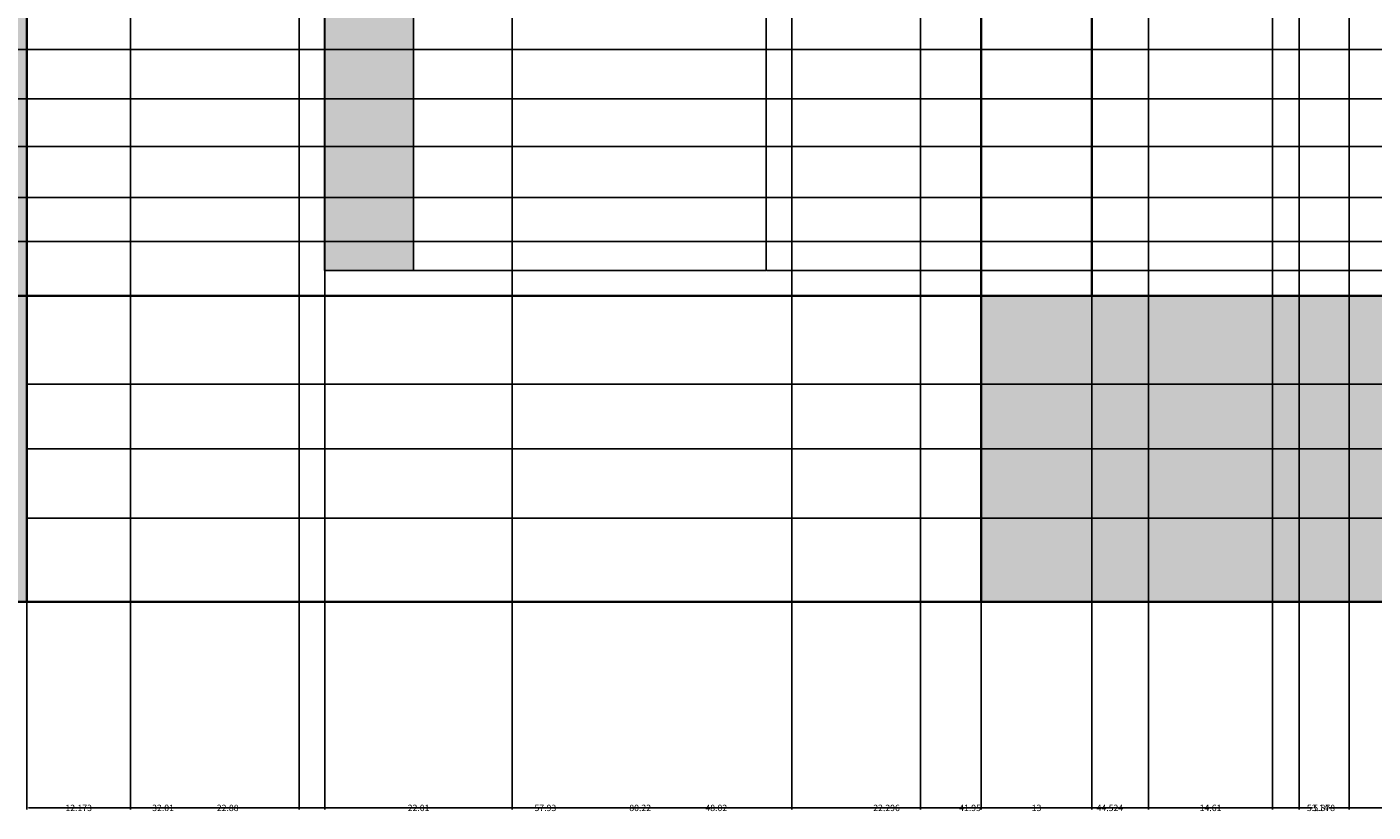
# Model space of a CAD drawing. Units: inches. Extents: x 62 to 566, y 66 to 528.
# Tile 11 of 20: x 284 to 443, y 66 to 158. Entities that reach past the tile are written whole.
import ezdxf

# ---------------------------------------------------------------- set-up
doc = ezdxf.new("R2010")
doc.units = ezdxf.units.IN
doc.header["$MEASUREMENT"] = 0
for name, color, linetype, lineweight in [('A-ANNO-DIMS', 2, 'Continuous', 18), ('A-DOOR', 4, 'Continuous', 25), ('A-ELEV', 7, 'Continuous', 35), ('A-FLOR-STRS', 2, 'Continuous', 25), ('A-WALL-PATT', 8, 'Continuous', 13)]:
    doc.layers.add(name, color=color, linetype=linetype, lineweight=lineweight)
doc.styles.get("Standard").update_dxf_attribs({"font": 'arial.ttf'})
doc.dimstyles.get("Standard").update_dxf_attribs({"dimtxt": 0.75, "dimasz": 0.18, "dimexe": 0.18, "dimexo": 0.0625, "dimgap": 0.09, "dimtad": 0, "dimtih": 1, "dimtoh": 1, "dimdec": 4, "dimzin": 0, "dimdsep": 46, "dimlunit": 4, "dimtxsty": 'Standard', "dimcen": 0.09, "dimadec": 0, "dimazin": 0, "dimtfac": 1, "dimtdec": 4, "dimtofl": 0, "dimtmove": 0, "dimatfit": 3, "dimfxl": 1, "dimtolj": 1, "dimtzin": 0, "dimarcsym": 0})

# ---------------------------------------------------------------- blocks, each defined once
blk = doc.blocks.new('*D9')
at = {"layer": 'A-ANNO-DIMS', "color": 0, "lineweight": -2, "transparency": 16777216}
for p, q in [((284.2, 271.35), (284.2, 65.94)), ((316.21, 126.31), (316.21, 65.94)), ((284.38, 66.12), (298.92, 66.12)), ((316.03, 66.12), (301.49, 66.12))]:
    blk.add_line(p, q, dxfattribs=at)
at = {"layer": 'A-ANNO-DIMS', "color": 0, "transparency": 16777216}
for points in [[(284.38, 66.15), (284.38, 66.09), (284.2, 66.12)], [(316.03, 66.15), (316.03, 66.09), (316.21, 66.12)]]:
    blk.add_solid(points, dxfattribs=at)
at = {"layer": 'Defpoints', "color": 0, "transparency": 16777216}
for p in [(284.2, 271.41), (316.21, 126.37), (316.21, 66.12)]:
    blk.add_point(p, dxfattribs=at)
at = {"layer": 'A-ANNO-DIMS', "color": 0, "transparency": 16777216, "insert": (300.21, 66.12), "char_height": 0.75, "attachment_point": 5}
blk.add_mtext('\\A1;32.01', dxfattribs=at)
blk = doc.blocks.new('*D10')
at = {"layer": 'A-ANNO-DIMS', "color": 0, "lineweight": -2, "transparency": 16777216}
for p, q in [((396.43, 271.35), (396.43, 65.94)), ((316.21, 126.31), (316.21, 65.94)), ((316.39, 66.12), (354.97, 66.12)), ((396.25, 66.12), (357.67, 66.12))]:
    blk.add_line(p, q, dxfattribs=at)
at = {"layer": 'A-ANNO-DIMS', "color": 0, "transparency": 16777216}
for points in [[(316.39, 66.15), (316.39, 66.09), (316.21, 66.12)], [(396.25, 66.15), (396.25, 66.09), (396.43, 66.12)]]:
    blk.add_solid(points, dxfattribs=at)
at = {"layer": 'Defpoints', "color": 0, "transparency": 16777216}
for p in [(396.43, 271.41), (316.21, 126.37), (396.43, 66.12)]:
    blk.add_point(p, dxfattribs=at)
at = {"layer": 'A-ANNO-DIMS', "color": 0, "transparency": 16777216, "insert": (356.32, 66.12), "char_height": 0.75, "attachment_point": 5}
blk.add_mtext('\\A1;80.22', dxfattribs=at)
blk = doc.blocks.new('*D11')
at = {"layer": 'A-ANNO-DIMS', "color": 0, "lineweight": -2, "transparency": 16777216}
for p, q in [((396.43, 271.35), (396.43, 65.94)), ((409.43, 126.31), (409.43, 65.94)), ((396.61, 66.12), (402.34, 66.12)), ((409.25, 66.12), (403.52, 66.12))]:
    blk.add_line(p, q, dxfattribs=at)
at = {"layer": 'A-ANNO-DIMS', "color": 0, "transparency": 16777216}
for points in [[(396.61, 66.15), (396.61, 66.09), (396.43, 66.12)], [(409.25, 66.15), (409.25, 66.09), (409.43, 66.12)]]:
    blk.add_solid(points, dxfattribs=at)
at = {"layer": 'Defpoints', "color": 0, "transparency": 16777216}
for p in [(396.43, 271.41), (409.43, 126.37), (409.43, 66.12)]:
    blk.add_point(p, dxfattribs=at)
at = {"layer": 'A-ANNO-DIMS', "color": 0, "transparency": 16777216, "insert": (402.93, 66.12), "char_height": 0.75, "attachment_point": 5}
blk.add_mtext('\\A1;13', dxfattribs=at)
blk = doc.blocks.new('*D12')
at = {"layer": 'A-ANNO-DIMS', "color": 0, "lineweight": -2, "transparency": 16777216}
for p, q in [((409.43, 126.31), (409.43, 65.94)), ((462.58, 126.31), (462.58, 65.94)), ((409.61, 66.12), (434.65, 66.12)), ((462.4, 66.12), (437.36, 66.12))]:
    blk.add_line(p, q, dxfattribs=at)
at = {"layer": 'A-ANNO-DIMS', "color": 0, "transparency": 16777216}
for points in [[(409.61, 66.15), (409.61, 66.09), (409.43, 66.12)], [(462.4, 66.15), (462.4, 66.09), (462.58, 66.12)]]:
    blk.add_solid(points, dxfattribs=at)
at = {"layer": 'Defpoints', "color": 0, "transparency": 16777216}
for p in [(409.43, 126.37), (462.58, 126.37), (462.58, 66.12)]:
    blk.add_point(p, dxfattribs=at)
at = {"layer": 'A-ANNO-DIMS', "color": 0, "transparency": 16777216, "insert": (436, 66.12), "char_height": 0.75, "attachment_point": 5}
blk.add_mtext('\\A1;53.14', dxfattribs=at)
blk = doc.blocks.new('*D40')
at = {"layer": 'A-ANNO-DIMS', "color": 0, "lineweight": -2, "transparency": 16777216}
for p, q in [((284.2, 445.04), (284.2, 65.94)), ((316.21, 417.64), (316.21, 65.94)), ((284.38, 66.12), (298.92, 66.12)), ((316.03, 66.12), (301.49, 66.12))]:
    blk.add_line(p, q, dxfattribs=at)
at = {"layer": 'A-ANNO-DIMS', "color": 0, "transparency": 16777216}
for points in [[(284.38, 66.15), (284.38, 66.09), (284.2, 66.12)], [(316.03, 66.15), (316.03, 66.09), (316.21, 66.12)]]:
    blk.add_solid(points, dxfattribs=at)
at = {"layer": 'Defpoints', "color": 0, "transparency": 16777216}
for p in [(284.2, 445.11), (316.21, 417.71), (316.21, 66.12)]:
    blk.add_point(p, dxfattribs=at)
at = {"layer": 'A-ANNO-DIMS', "color": 0, "transparency": 16777216, "insert": (300.21, 66.12), "char_height": 0.75, "attachment_point": 5}
blk.add_mtext('\\A1;32.01', dxfattribs=at)
blk = doc.blocks.new('*D41')
at = {"layer": 'A-ANNO-DIMS', "color": 0, "lineweight": -2, "transparency": 16777216}
for p, q in [((316.21, 417.64), (316.21, 65.94)), ((374.14, 417.64), (374.14, 65.94)), ((316.39, 66.12), (343.82, 66.12)), ((373.96, 66.12), (346.53, 66.12))]:
    blk.add_line(p, q, dxfattribs=at)
at = {"layer": 'A-ANNO-DIMS', "color": 0, "transparency": 16777216}
for points in [[(316.39, 66.15), (316.39, 66.09), (316.21, 66.12)], [(373.96, 66.15), (373.96, 66.09), (374.14, 66.12)]]:
    blk.add_solid(points, dxfattribs=at)
at = {"layer": 'Defpoints', "color": 0, "transparency": 16777216}
for p in [(316.21, 417.71), (374.14, 417.71), (374.14, 66.12)]:
    blk.add_point(p, dxfattribs=at)
at = {"layer": 'A-ANNO-DIMS', "color": 0, "transparency": 16777216, "insert": (345.17, 66.12), "char_height": 0.75, "attachment_point": 5}
blk.add_mtext('\\A1;57.93', dxfattribs=at)
blk = doc.blocks.new('*D42')
at = {"layer": 'A-ANNO-DIMS', "color": 0, "lineweight": -2, "transparency": 16777216}
for p, q in [((416.08, 445.04), (416.08, 65.94)), ((374.14, 417.64), (374.14, 65.94)), ((374.32, 66.12), (393.74, 66.12)), ((415.9, 66.12), (396.48, 66.12))]:
    blk.add_line(p, q, dxfattribs=at)
at = {"layer": 'A-ANNO-DIMS', "color": 0, "transparency": 16777216}
for points in [[(374.32, 66.15), (374.32, 66.09), (374.14, 66.12)], [(415.9, 66.15), (415.9, 66.09), (416.08, 66.12)]]:
    blk.add_solid(points, dxfattribs=at)
at = {"layer": 'Defpoints', "color": 0, "transparency": 16777216}
for p in [(416.08, 445.11), (374.14, 417.71), (416.08, 66.12)]:
    blk.add_point(p, dxfattribs=at)
at = {"layer": 'A-ANNO-DIMS', "color": 0, "transparency": 16777216, "insert": (395.11, 66.12), "char_height": 0.75, "attachment_point": 5}
blk.add_mtext('\\A1;41.95', dxfattribs=at)
blk = doc.blocks.new('*D43')
at = {"layer": 'A-ANNO-DIMS', "color": 0, "lineweight": -2, "transparency": 16777216}
for p, q in [((416.08, 445.04), (416.08, 65.94)), ((430.69, 445.04), (430.69, 65.94)), ((416.26, 66.12), (422.14, 66.12)), ((430.51, 66.12), (424.64, 66.12))]:
    blk.add_line(p, q, dxfattribs=at)
at = {"layer": 'A-ANNO-DIMS', "color": 0, "transparency": 16777216}
for points in [[(416.26, 66.15), (416.26, 66.09), (416.08, 66.12)], [(430.51, 66.15), (430.51, 66.09), (430.69, 66.12)]]:
    blk.add_solid(points, dxfattribs=at)
at = {"layer": 'Defpoints', "color": 0, "transparency": 16777216}
for p in [(416.08, 445.11), (430.69, 445.11), (430.69, 66.12)]:
    blk.add_point(p, dxfattribs=at)
at = {"layer": 'A-ANNO-DIMS', "color": 0, "transparency": 16777216, "insert": (423.39, 66.12), "char_height": 0.75, "attachment_point": 5}
blk.add_mtext('\\A1;14.61', dxfattribs=at)
blk = doc.blocks.new('*D57')
at = {"layer": 'A-ANNO-DIMS', "color": 0, "lineweight": -2, "transparency": 16777216}
for p, q in [((316.21, 126.31), (316.21, 65.94)), ((284.2, 90.31), (284.2, 65.94)), ((284.38, 66.12), (298.92, 66.12)), ((316.03, 66.12), (301.49, 66.12))]:
    blk.add_line(p, q, dxfattribs=at)
at = {"layer": 'A-ANNO-DIMS', "color": 0, "transparency": 16777216}
for points in [[(284.38, 66.15), (284.38, 66.09), (284.2, 66.12)], [(316.03, 66.15), (316.03, 66.09), (316.21, 66.12)]]:
    blk.add_solid(points, dxfattribs=at)
at = {"layer": 'Defpoints', "color": 0, "transparency": 16777216}
for p in [(316.21, 126.37), (284.2, 90.37), (316.21, 66.12)]:
    blk.add_point(p, dxfattribs=at)
at = {"layer": 'A-ANNO-DIMS', "color": 0, "transparency": 16777216, "insert": (300.21, 66.12), "char_height": 0.75, "attachment_point": 5}
blk.add_mtext('\\A1;32.01', dxfattribs=at)
blk = doc.blocks.new('*D58')
at = {"layer": 'A-ANNO-DIMS', "color": 0, "lineweight": -2, "transparency": 16777216}
for p, q in [((316.21, 126.31), (316.21, 65.94)), ((374.14, 126.31), (374.14, 65.94)), ((316.39, 66.12), (343.82, 66.12)), ((373.96, 66.12), (346.53, 66.12))]:
    blk.add_line(p, q, dxfattribs=at)
at = {"layer": 'A-ANNO-DIMS', "color": 0, "transparency": 16777216}
for points in [[(316.39, 66.15), (316.39, 66.09), (316.21, 66.12)], [(373.96, 66.15), (373.96, 66.09), (374.14, 66.12)]]:
    blk.add_solid(points, dxfattribs=at)
at = {"layer": 'Defpoints', "color": 0, "transparency": 16777216}
for p in [(316.21, 126.37), (374.14, 126.37), (374.14, 66.12)]:
    blk.add_point(p, dxfattribs=at)
at = {"layer": 'A-ANNO-DIMS', "color": 0, "transparency": 16777216, "insert": (345.17, 66.12), "char_height": 0.75, "attachment_point": 5}
blk.add_mtext('\\A1;57.93', dxfattribs=at)
blk = doc.blocks.new('*D59')
at = {"layer": 'A-ANNO-DIMS', "color": 0, "lineweight": -2, "transparency": 16777216}
for p, q in [((374.14, 126.31), (374.14, 65.94)), ((396.43, 90.31), (396.43, 65.94)), ((374.32, 66.12), (383.63, 66.12)), ((396.25, 66.12), (386.94, 66.12))]:
    blk.add_line(p, q, dxfattribs=at)
at = {"layer": 'A-ANNO-DIMS', "color": 0, "transparency": 16777216}
for points in [[(374.32, 66.15), (374.32, 66.09), (374.14, 66.12)], [(396.25, 66.15), (396.25, 66.09), (396.43, 66.12)]]:
    blk.add_solid(points, dxfattribs=at)
at = {"layer": 'Defpoints', "color": 0, "transparency": 16777216}
for p in [(374.14, 126.37), (396.43, 90.37), (396.43, 66.12)]:
    blk.add_point(p, dxfattribs=at)
at = {"layer": 'A-ANNO-DIMS', "color": 0, "transparency": 16777216, "insert": (385.29, 66.12), "char_height": 0.75, "attachment_point": 5}
blk.add_mtext('\\A1;22.296', dxfattribs=at)
blk = doc.blocks.new('*D60')
at = {"layer": 'A-ANNO-DIMS', "color": 0, "lineweight": -2, "transparency": 16777216}
for p, q in [((409.43, 126.31), (409.43, 65.94)), ((396.43, 90.31), (396.43, 65.94)), ((396.61, 66.12), (402.34, 66.12)), ((409.25, 66.12), (403.52, 66.12))]:
    blk.add_line(p, q, dxfattribs=at)
at = {"layer": 'A-ANNO-DIMS', "color": 0, "transparency": 16777216}
for points in [[(396.61, 66.15), (396.61, 66.09), (396.43, 66.12)], [(409.25, 66.15), (409.25, 66.09), (409.43, 66.12)]]:
    blk.add_solid(points, dxfattribs=at)
at = {"layer": 'Defpoints', "color": 0, "transparency": 16777216}
for p in [(409.43, 126.37), (396.43, 90.37), (409.43, 66.12)]:
    blk.add_point(p, dxfattribs=at)
at = {"layer": 'A-ANNO-DIMS', "color": 0, "transparency": 16777216, "insert": (402.93, 66.12), "char_height": 0.75, "attachment_point": 5}
blk.add_mtext('\\A1;13', dxfattribs=at)
blk = doc.blocks.new('*D65')
at = {"layer": 'A-ANNO-DIMS', "color": 0, "lineweight": -2, "transparency": 16777216}
for p, q in [((396.5, 100.2), (564.47, 100.2)), ((564.29, 100.02), (564.29, 95.76)), ((564.29, 90.55), (564.29, 94.81)), ((396.5, 90.37), (564.47, 90.37))]:
    blk.add_line(p, q, dxfattribs=at)
at = {"layer": 'A-ANNO-DIMS', "color": 0, "transparency": 16777216}
for points in [[(564.26, 100.02), (564.32, 100.02), (564.29, 100.2)], [(564.26, 90.55), (564.32, 90.55), (564.29, 90.37)]]:
    blk.add_solid(points, dxfattribs=at)
at = {"layer": 'Defpoints', "color": 0, "transparency": 16777216}
for p in [(396.43, 100.2), (564.29, 100.2), (396.43, 90.37)]:
    blk.add_point(p, dxfattribs=at)
at = {"layer": 'A-ANNO-DIMS', "color": 0, "transparency": 16777216, "insert": (564.29, 95.28), "char_height": 0.75, "attachment_point": 5}
blk.add_mtext('\\A1;9.831', dxfattribs=at)
blk = doc.blocks.new('*D66')
at = {"layer": 'A-ANNO-DIMS', "color": 0, "lineweight": -2, "transparency": 16777216}
for p, q in [((396.5, 108.37), (564.47, 108.37)), ((564.29, 108.19), (564.29, 104.76)), ((564.29, 100.38), (564.29, 103.81)), ((396.5, 100.2), (564.47, 100.2))]:
    blk.add_line(p, q, dxfattribs=at)
at = {"layer": 'A-ANNO-DIMS', "color": 0, "transparency": 16777216}
for points in [[(564.26, 108.19), (564.32, 108.19), (564.29, 108.37)], [(564.26, 100.38), (564.32, 100.38), (564.29, 100.2)]]:
    blk.add_solid(points, dxfattribs=at)
at = {"layer": 'Defpoints', "color": 0, "transparency": 16777216}
for p in [(396.43, 108.37), (564.29, 108.37), (396.43, 100.2)]:
    blk.add_point(p, dxfattribs=at)
at = {"layer": 'A-ANNO-DIMS', "color": 0, "transparency": 16777216, "insert": (564.29, 104.28), "char_height": 0.75, "attachment_point": 5}
blk.add_mtext('\\A1;8.169', dxfattribs=at)
blk = doc.blocks.new('*D67')
at = {"layer": 'A-ANNO-DIMS', "color": 0, "lineweight": -2, "transparency": 16777216}
for p, q in [((396.5, 115.97), (564.47, 115.97)), ((564.29, 115.79), (564.29, 112.64)), ((564.29, 108.55), (564.29, 111.69)), ((396.5, 108.37), (564.47, 108.37))]:
    blk.add_line(p, q, dxfattribs=at)
at = {"layer": 'A-ANNO-DIMS', "color": 0, "transparency": 16777216}
for points in [[(564.26, 115.79), (564.32, 115.79), (564.29, 115.97)], [(564.26, 108.55), (564.32, 108.55), (564.29, 108.37)]]:
    blk.add_solid(points, dxfattribs=at)
at = {"layer": 'Defpoints', "color": 0, "transparency": 16777216}
for p in [(396.43, 115.97), (564.29, 115.97), (396.43, 108.37)]:
    blk.add_point(p, dxfattribs=at)
at = {"layer": 'A-ANNO-DIMS', "color": 0, "transparency": 16777216, "insert": (564.29, 112.17), "char_height": 0.75, "attachment_point": 5}
blk.add_mtext('\\A1;7.599', dxfattribs=at)
blk = doc.blocks.new('*D68')
at = {"layer": 'A-ANNO-DIMS', "color": 0, "lineweight": -2, "transparency": 16777216}
for p, q in [((374.2, 126.37), (564.47, 126.37)), ((564.29, 126.19), (564.29, 121.64)), ((564.29, 116.15), (564.29, 120.69)), ((396.5, 115.97), (564.47, 115.97))]:
    blk.add_line(p, q, dxfattribs=at)
at = {"layer": 'A-ANNO-DIMS', "color": 0, "transparency": 16777216}
for points in [[(564.26, 126.19), (564.32, 126.19), (564.29, 126.37)], [(564.26, 116.15), (564.32, 116.15), (564.29, 115.97)]]:
    blk.add_solid(points, dxfattribs=at)
at = {"layer": 'Defpoints', "color": 0, "transparency": 16777216}
for p in [(374.14, 126.37), (564.29, 126.37), (396.43, 115.97)]:
    blk.add_point(p, dxfattribs=at)
at = {"layer": 'A-ANNO-DIMS', "color": 0, "transparency": 16777216, "insert": (564.29, 121.17), "char_height": 0.75, "attachment_point": 5}
blk.add_mtext('\\A1;10.401', dxfattribs=at)
blk = doc.blocks.new('*D69')
at = {"layer": 'A-ANNO-DIMS', "color": 0, "lineweight": -2, "transparency": 16777216}
for p, q in [((371.2, 129.37), (564.47, 129.37)), ((564.29, 129.19), (564.29, 128.34)), ((564.29, 126.55), (564.29, 127.4)), ((374.2, 126.37), (564.47, 126.37))]:
    blk.add_line(p, q, dxfattribs=at)
at = {"layer": 'A-ANNO-DIMS', "color": 0, "transparency": 16777216}
for points in [[(564.26, 129.19), (564.32, 129.19), (564.29, 129.37)], [(564.26, 126.55), (564.32, 126.55), (564.29, 126.37)]]:
    blk.add_solid(points, dxfattribs=at)
at = {"layer": 'Defpoints', "color": 0, "transparency": 16777216}
for p in [(371.14, 129.37), (564.29, 129.37), (374.14, 126.37)]:
    blk.add_point(p, dxfattribs=at)
at = {"layer": 'A-ANNO-DIMS', "color": 0, "transparency": 16777216, "insert": (564.29, 127.87), "char_height": 0.75, "attachment_point": 5}
blk.add_mtext('\\A1;3', dxfattribs=at)
blk = doc.blocks.new('*D70')
at = {"layer": 'A-ANNO-DIMS', "color": 0, "lineweight": -2, "transparency": 16777216}
for p, q in [((329.73, 219.73), (564.47, 219.73)), ((564.29, 219.55), (564.29, 175.02)), ((564.29, 129.55), (564.29, 174.08)), ((371.2, 129.37), (564.47, 129.37))]:
    blk.add_line(p, q, dxfattribs=at)
at = {"layer": 'A-ANNO-DIMS', "color": 0, "transparency": 16777216}
for points in [[(564.26, 219.55), (564.32, 219.55), (564.29, 219.73)], [(564.26, 129.55), (564.32, 129.55), (564.29, 129.37)]]:
    blk.add_solid(points, dxfattribs=at)
at = {"layer": 'Defpoints', "color": 0, "transparency": 16777216}
for p in [(329.67, 219.73), (564.29, 219.73), (371.14, 129.37)]:
    blk.add_point(p, dxfattribs=at)
at = {"layer": 'A-ANNO-DIMS', "color": 0, "transparency": 16777216, "insert": (564.29, 174.55), "char_height": 0.75, "attachment_point": 5}
blk.add_mtext('\\A1;90.36', dxfattribs=at)
blk = doc.blocks.new('*D73')
at = {"layer": 'A-ANNO-DIMS', "color": 0, "lineweight": -2, "transparency": 16777216}
for p, q in [((316.15, 236.66), (63.47, 236.66)), ((63.65, 236.48), (63.65, 181.99)), ((63.65, 126.55), (63.65, 181.04)), ((316.15, 126.37), (63.47, 126.37))]:
    blk.add_line(p, q, dxfattribs=at)
at = {"layer": 'A-ANNO-DIMS', "color": 0, "transparency": 16777216}
for points in [[(63.62, 236.48), (63.68, 236.48), (63.65, 236.66)], [(63.62, 126.55), (63.68, 126.55), (63.65, 126.37)]]:
    blk.add_solid(points, dxfattribs=at)
at = {"layer": 'Defpoints', "color": 0, "transparency": 16777216}
for p in [(63.65, 236.66), (316.21, 236.66), (316.21, 126.37)]:
    blk.add_point(p, dxfattribs=at)
at = {"layer": 'A-ANNO-DIMS', "color": 0, "transparency": 16777216, "insert": (63.65, 181.52), "char_height": 0.75, "attachment_point": 5}
blk.add_mtext('\\A1;110.3', dxfattribs=at)
blk = doc.blocks.new('*D82')
at = {"layer": 'A-ANNO-DIMS', "color": 0, "lineweight": -2, "transparency": 16777216}
for p, q in [((296.38, 279.98), (296.38, 65.94)), ((284.2, 271.35), (284.2, 65.94)), ((284.38, 66.12), (288.68, 66.12)), ((296.2, 66.12), (291.9, 66.12))]:
    blk.add_line(p, q, dxfattribs=at)
at = {"layer": 'A-ANNO-DIMS', "color": 0, "transparency": 16777216}
for points in [[(284.38, 66.15), (284.38, 66.09), (284.2, 66.12)], [(296.2, 66.15), (296.2, 66.09), (296.38, 66.12)]]:
    blk.add_solid(points, dxfattribs=at)
at = {"layer": 'Defpoints', "color": 0, "transparency": 16777216}
for p in [(296.38, 280.04), (284.2, 271.41), (296.38, 66.12)]:
    blk.add_point(p, dxfattribs=at)
at = {"layer": 'A-ANNO-DIMS', "color": 0, "transparency": 16777216, "insert": (290.29, 66.12), "char_height": 0.75, "attachment_point": 5}
blk.add_mtext('\\A1;12.173', dxfattribs=at)
blk = doc.blocks.new('*D83')
at = {"layer": 'A-ANNO-DIMS', "color": 0, "lineweight": -2, "transparency": 16777216}
for p, q in [((296.38, 279.98), (296.38, 65.94)), ((319.25, 279.98), (319.25, 65.94)), ((296.56, 66.12), (306.45, 66.12)), ((319.07, 66.12), (309.18, 66.12))]:
    blk.add_line(p, q, dxfattribs=at)
at = {"layer": 'A-ANNO-DIMS', "color": 0, "transparency": 16777216}
for points in [[(296.56, 66.15), (296.56, 66.09), (296.38, 66.12)], [(319.07, 66.15), (319.07, 66.09), (319.25, 66.12)]]:
    blk.add_solid(points, dxfattribs=at)
at = {"layer": 'Defpoints', "color": 0, "transparency": 16777216}
for p in [(296.38, 280.04), (319.25, 280.04), (319.25, 66.12)]:
    blk.add_point(p, dxfattribs=at)
at = {"layer": 'A-ANNO-DIMS', "color": 0, "transparency": 16777216, "insert": (307.81, 66.12), "char_height": 0.75, "attachment_point": 5}
blk.add_mtext('\\A1;22.88', dxfattribs=at)
blk = doc.blocks.new('*D84')
at = {"layer": 'A-ANNO-DIMS', "color": 0, "lineweight": -2, "transparency": 16777216}
for p, q in [((319.25, 279.98), (319.25, 65.94)), ((341.26, 279.98), (341.26, 65.94)), ((319.43, 66.12), (328.97, 66.12)), ((341.08, 66.12), (331.55, 66.12))]:
    blk.add_line(p, q, dxfattribs=at)
at = {"layer": 'A-ANNO-DIMS', "color": 0, "transparency": 16777216}
for points in [[(319.43, 66.15), (319.43, 66.09), (319.25, 66.12)], [(341.08, 66.15), (341.08, 66.09), (341.26, 66.12)]]:
    blk.add_solid(points, dxfattribs=at)
at = {"layer": 'Defpoints', "color": 0, "transparency": 16777216}
for p in [(319.25, 280.04), (341.26, 280.04), (341.26, 66.12)]:
    blk.add_point(p, dxfattribs=at)
at = {"layer": 'A-ANNO-DIMS', "color": 0, "transparency": 16777216, "insert": (330.26, 66.12), "char_height": 0.75, "attachment_point": 5}
blk.add_mtext('\\A1;22.01', dxfattribs=at)
blk = doc.blocks.new('*D85')
at = {"layer": 'A-ANNO-DIMS', "color": 0, "lineweight": -2, "transparency": 16777216}
for p, q in [((389.29, 281.45), (389.29, 65.94)), ((341.26, 279.98), (341.26, 65.94)), ((341.44, 66.12), (363.91, 66.12)), ((389.11, 66.12), (366.64, 66.12))]:
    blk.add_line(p, q, dxfattribs=at)
at = {"layer": 'A-ANNO-DIMS', "color": 0, "transparency": 16777216}
for points in [[(341.44, 66.15), (341.44, 66.09), (341.26, 66.12)], [(389.11, 66.15), (389.11, 66.09), (389.29, 66.12)]]:
    blk.add_solid(points, dxfattribs=at)
at = {"layer": 'Defpoints', "color": 0, "transparency": 16777216}
for p in [(389.29, 281.51), (341.26, 280.04), (389.29, 66.12)]:
    blk.add_point(p, dxfattribs=at)
at = {"layer": 'A-ANNO-DIMS', "color": 0, "transparency": 16777216, "insert": (365.27, 66.12), "char_height": 0.75, "attachment_point": 5}
blk.add_mtext('\\A1;48.02', dxfattribs=at)
blk = doc.blocks.new('*D86')
at = {"layer": 'A-ANNO-DIMS', "color": 0, "lineweight": -2, "transparency": 16777216}
for p, q in [((389.29, 281.45), (389.29, 65.94)), ((433.81, 281.45), (433.81, 65.94)), ((389.47, 66.12), (409.89, 66.12)), ((433.63, 66.12), (413.21, 66.12))]:
    blk.add_line(p, q, dxfattribs=at)
at = {"layer": 'A-ANNO-DIMS', "color": 0, "transparency": 16777216}
for points in [[(389.47, 66.15), (389.47, 66.09), (389.29, 66.12)], [(433.63, 66.15), (433.63, 66.09), (433.81, 66.12)]]:
    blk.add_solid(points, dxfattribs=at)
at = {"layer": 'Defpoints', "color": 0, "transparency": 16777216}
for p in [(389.29, 281.51), (433.81, 281.51), (433.81, 66.12)]:
    blk.add_point(p, dxfattribs=at)
at = {"layer": 'A-ANNO-DIMS', "color": 0, "transparency": 16777216, "insert": (411.55, 66.12), "char_height": 0.75, "attachment_point": 5}
blk.add_mtext('\\A1;44.524', dxfattribs=at)
blk = doc.blocks.new('*D87')
at = {"layer": 'A-ANNO-DIMS', "color": 0, "lineweight": -2, "transparency": 16777216}
for p, q in [((433.81, 281.45), (433.81, 65.94)), ((439.69, 271.35), (439.69, 65.94)), ((433.99, 66.12), (435.39, 66.12)), ((439.51, 66.12), (438.11, 66.12))]:
    blk.add_line(p, q, dxfattribs=at)
at = {"layer": 'A-ANNO-DIMS', "color": 0, "transparency": 16777216}
for points in [[(433.99, 66.15), (433.99, 66.09), (433.81, 66.12)], [(439.51, 66.15), (439.51, 66.09), (439.69, 66.12)]]:
    blk.add_solid(points, dxfattribs=at)
at = {"layer": 'Defpoints', "color": 0, "transparency": 16777216}
for p in [(433.81, 281.51), (439.69, 271.41), (439.69, 66.12)]:
    blk.add_point(p, dxfattribs=at)
at = {"layer": 'A-ANNO-DIMS', "color": 0, "transparency": 16777216, "insert": (436.75, 66.12), "char_height": 0.75, "attachment_point": 5}
blk.add_mtext('\\A1;5.878', dxfattribs=at)
blk = doc.blocks.new('*D116')
at = {"layer": 'A-ANNO-DIMS', "color": 0, "lineweight": -2, "transparency": 16777216}
for p, q in [((267.86, 132.79), (564.47, 132.79)), ((564.29, 132.61), (564.29, 130.05)), ((564.29, 126.55), (564.29, 129.11)), ((272.12, 126.37), (564.47, 126.37))]:
    blk.add_line(p, q, dxfattribs=at)
at = {"layer": 'A-ANNO-DIMS', "color": 0, "transparency": 16777216}
for points in [[(564.26, 132.61), (564.32, 132.61), (564.29, 132.79)], [(564.26, 126.55), (564.32, 126.55), (564.29, 126.37)]]:
    blk.add_solid(points, dxfattribs=at)
at = {"layer": 'Defpoints', "color": 0, "transparency": 16777216}
for p in [(267.79, 132.79), (564.29, 132.79), (272.06, 126.37)]:
    blk.add_point(p, dxfattribs=at)
at = {"layer": 'A-ANNO-DIMS', "color": 0, "transparency": 16777216, "insert": (564.29, 129.58), "char_height": 0.75, "attachment_point": 5}
blk.add_mtext('\\A1;6.426', dxfattribs=at)
blk = doc.blocks.new('*D117')
at = {"layer": 'A-ANNO-DIMS', "color": 0, "lineweight": -2, "transparency": 16777216}
for p, q in [((267.86, 137.96), (564.47, 137.96)), ((564.29, 137.78), (564.29, 135.85)), ((564.29, 132.97), (564.29, 134.91)), ((267.86, 132.79), (564.47, 132.79))]:
    blk.add_line(p, q, dxfattribs=at)
at = {"layer": 'A-ANNO-DIMS', "color": 0, "transparency": 16777216}
for points in [[(564.26, 137.78), (564.32, 137.78), (564.29, 137.96)], [(564.26, 132.97), (564.32, 132.97), (564.29, 132.79)]]:
    blk.add_solid(points, dxfattribs=at)
at = {"layer": 'Defpoints', "color": 0, "transparency": 16777216}
for p in [(267.79, 137.96), (564.29, 137.96), (267.79, 132.79)]:
    blk.add_point(p, dxfattribs=at)
at = {"layer": 'A-ANNO-DIMS', "color": 0, "transparency": 16777216, "insert": (564.29, 135.38), "char_height": 0.75, "attachment_point": 5}
blk.add_mtext('\\A1;5.17', dxfattribs=at)
blk = doc.blocks.new('*D118')
at = {"layer": 'A-ANNO-DIMS', "color": 0, "lineweight": -2, "transparency": 16777216}
for p, q in [((267.86, 143.95), (564.47, 143.95)), ((564.29, 143.77), (564.29, 141.43)), ((564.29, 138.14), (564.29, 140.49)), ((267.86, 137.96), (564.47, 137.96))]:
    blk.add_line(p, q, dxfattribs=at)
at = {"layer": 'A-ANNO-DIMS', "color": 0, "transparency": 16777216}
for points in [[(564.26, 143.77), (564.32, 143.77), (564.29, 143.95)], [(564.26, 138.14), (564.32, 138.14), (564.29, 137.96)]]:
    blk.add_solid(points, dxfattribs=at)
at = {"layer": 'Defpoints', "color": 0, "transparency": 16777216}
for p in [(267.79, 143.95), (564.29, 143.95), (267.79, 137.96)]:
    blk.add_point(p, dxfattribs=at)
at = {"layer": 'A-ANNO-DIMS', "color": 0, "transparency": 16777216, "insert": (564.29, 140.96), "char_height": 0.75, "attachment_point": 5}
blk.add_mtext('\\A1;5.986', dxfattribs=at)
blk = doc.blocks.new('*D119')
at = {"layer": 'A-ANNO-DIMS', "color": 0, "lineweight": -2, "transparency": 16777216}
for p, q in [((267.86, 149.57), (564.47, 149.57)), ((564.29, 149.39), (564.29, 147.24)), ((564.29, 144.13), (564.29, 146.29)), ((267.86, 143.95), (564.47, 143.95))]:
    blk.add_line(p, q, dxfattribs=at)
at = {"layer": 'A-ANNO-DIMS', "color": 0, "transparency": 16777216}
for points in [[(564.26, 149.39), (564.32, 149.39), (564.29, 149.57)], [(564.26, 144.13), (564.32, 144.13), (564.29, 143.95)]]:
    blk.add_solid(points, dxfattribs=at)
at = {"layer": 'Defpoints', "color": 0, "transparency": 16777216}
for p in [(267.79, 149.57), (564.29, 149.57), (267.79, 143.95)]:
    blk.add_point(p, dxfattribs=at)
at = {"layer": 'A-ANNO-DIMS', "color": 0, "transparency": 16777216, "insert": (564.29, 146.76), "char_height": 0.75, "attachment_point": 5}
blk.add_mtext('\\A1;5.624', dxfattribs=at)
blk = doc.blocks.new('*D120')
at = {"layer": 'A-ANNO-DIMS', "color": 0, "lineweight": -2, "transparency": 16777216}
for p, q in [((267.86, 155.38), (564.47, 155.38)), ((564.29, 155.2), (564.29, 152.95)), ((564.29, 149.75), (564.29, 152)), ((267.86, 149.57), (564.47, 149.57))]:
    blk.add_line(p, q, dxfattribs=at)
at = {"layer": 'A-ANNO-DIMS', "color": 0, "transparency": 16777216}
for points in [[(564.26, 155.2), (564.32, 155.2), (564.29, 155.38)], [(564.26, 149.75), (564.32, 149.75), (564.29, 149.57)]]:
    blk.add_solid(points, dxfattribs=at)
at = {"layer": 'Defpoints', "color": 0, "transparency": 16777216}
for p in [(267.79, 155.38), (564.29, 155.38), (267.79, 149.57)]:
    blk.add_point(p, dxfattribs=at)
at = {"layer": 'A-ANNO-DIMS', "color": 0, "transparency": 16777216, "insert": (564.29, 152.48), "char_height": 0.75, "attachment_point": 5}
blk.add_mtext('\\A1;5.805', dxfattribs=at)
blk = doc.blocks.new('*D121')
at = {"layer": 'A-ANNO-DIMS', "color": 0, "lineweight": -2, "transparency": 16777216}
for p, q in [((272.12, 160.35), (564.47, 160.35)), ((564.29, 160.17), (564.29, 158.34)), ((564.29, 155.56), (564.29, 157.39)), ((267.86, 155.38), (564.47, 155.38))]:
    blk.add_line(p, q, dxfattribs=at)
at = {"layer": 'A-ANNO-DIMS', "color": 0, "transparency": 16777216}
for points in [[(564.26, 160.17), (564.32, 160.17), (564.29, 160.35)], [(564.26, 155.56), (564.32, 155.56), (564.29, 155.38)]]:
    blk.add_solid(points, dxfattribs=at)
at = {"layer": 'Defpoints', "color": 0, "transparency": 16777216}
for p in [(272.06, 160.35), (564.29, 160.35), (267.79, 155.38)]:
    blk.add_point(p, dxfattribs=at)
at = {"layer": 'A-ANNO-DIMS', "color": 0, "transparency": 16777216, "insert": (564.29, 157.87), "char_height": 0.75, "attachment_point": 5}
blk.add_mtext('\\A1;4.975', dxfattribs=at)

msp = doc.modelspace()

# ---------------------------------------------------------------- hatches: boundary and pattern name
at = {"layer": 'A-WALL-PATT'}
h = msp.add_hatch(dxfattribs=at)
h.set_pattern_fill('ANSI36', color=256, scale=8.8)
h.paths.add_polyline_path([(217.2752, 420.597), (169.0431, 420.597), (169.0431, 126.3686), (217.2752, 126.3686), (217.2752, 129.0504), (217.2752, 271.4128), (217.2752, 295.4128), (217.2752, 307.4128)])
h.paths.add_polyline_path([(282.3509, 501.0423), (125.9418, 501.0423), (125.9418, 465.0423), (282.3509, 465.0423)])
h.paths.add_polyline_path([(209.709, 476.6506), (202.045, 476.6506), (202.045, 493.7764), (209.709, 493.7764)], flags=16)
h.paths.add_polyline_path([(193.9913, 476.6506), (186.3273, 476.6506), (186.3273, 493.7764), (193.9913, 493.7764)], flags=16)
h.paths.add_polyline_path([(177.9243, 476.6506), (170.2603, 476.6506), (170.2603, 493.7764), (177.9243, 493.7764)], flags=16)
h.paths.add_polyline_path([(163.2545, 476.3015), (155.5905, 476.3015), (155.5905, 493.4274), (163.2545, 493.4274)], flags=16)
h.paths.add_polyline_path([(148.2354, 476.3015), (140.5713, 476.3015), (140.5713, 493.4274), (148.2354, 493.4274)], flags=16)
h.paths.add_polyline_path([(284.2021, 126.3686), (87.8962, 126.3686), (87.8962, 114.3686), (87.8962, 90.3686), (284.2021, 90.3686)])
h.paths.add_polyline_path([(474.1214, 126.3686), (396.433, 126.3686), (396.433, 90.3686), (474.1214, 90.3686)])
h = msp.add_hatch(color=256, dxfattribs=at)
h.dxf.hatch_style = 1
h.paths.add_polyline_path([(416.0836, 501.0423), (282.3509, 501.0423), (282.3509, 465.0423), (416.0836, 465.0423)])
h.paths.add_polyline_path([(284.2021, 420.597), (272.0586, 420.597), (272.0586, 309.5388), (272.0586, 307.4128), (284.2021, 307.4128)], flags=17)
h.paths.add_polyline_path([(284.2021, 445.1064), (142.3851, 445.1064), (142.3851, 414.3686), (142.3851, 270.3686), (142.3851, 126.3686), (163.6548, 126.3686), (163.6548, 270.5016), (163.6548, 414.5016), (163.6548, 427.4752), (284.2021, 427.4752)])
h.paths.add_polyline_path([(235.4641, 297.1682), (227.8001, 297.1682), (227.8001, 280.0423), (235.4641, 280.0423)], flags=17)
h.paths.add_polyline_path([(255.6783, 297.1682), (248.0143, 297.1682), (248.0143, 280.0423), (255.6783, 280.0423)], flags=17)
h.paths.add_polyline_path([(278.1067, 297.1682), (270.4427, 297.1682), (270.4427, 280.0423), (278.1067, 280.0423)], flags=17)
h.paths.add_polyline_path([(304.0395, 297.1682), (296.3755, 297.1682), (296.3755, 280.0423), (304.0395, 280.0423)])
h.paths.add_polyline_path([(326.9183, 297.1682), (319.2543, 297.1682), (319.2543, 280.0423), (326.9183, 280.0423)])
h.paths.add_polyline_path([(348.9262, 297.1682), (341.2622, 297.1682), (341.2622, 280.0423), (348.9262, 280.0423)])
h.paths.add_polyline_path([(433.8102, 284.9607), (389.2857, 284.9607), (389.2857, 281.5119), (433.8102, 281.5119)])
h.paths.add_polyline_path([(433.8102, 291.6038), (389.2857, 291.6038), (389.2857, 288.155), (433.8102, 288.155)])
h.paths.add_polyline_path([(433.8102, 298.3985), (389.2857, 298.3985), (389.2857, 294.9497), (433.8102, 294.9497)])
h.paths.add_polyline_path([(433.1636, 317.4388), (403.5849, 317.4388), (403.5849, 311.4736), (433.1636, 311.4736)])
h.paths.add_polyline_path([(433.1636, 329.0982), (403.5849, 329.0982), (403.5849, 323.1329), (433.1636, 323.1329)])
h.paths.add_polyline_path([(433.1636, 340.4863), (403.5849, 340.4863), (403.5849, 334.5211), (433.1636, 334.5211)])
h.paths.add_polyline_path([(284.2021, 271.4128), (272.0586, 271.4128), (272.0586, 160.3545), (272.0586, 126.3686), (284.2021, 126.3686)])
h.paths.add_polyline_path([(267.7931, 158.101), (220.5897, 158.101), (220.5897, 155.3799), (267.7931, 155.3799)], flags=17)
h.paths.add_polyline_path([(267.7931, 152.296), (220.5897, 152.296), (220.5897, 149.5749), (267.7931, 149.5749)], flags=17)
h.paths.add_polyline_path([(267.7931, 146.6724), (220.5897, 146.6724), (220.5897, 143.9513), (267.7931, 143.9513)], flags=17)
h.paths.add_polyline_path([(267.7931, 140.686), (220.5897, 140.686), (220.5897, 137.9649), (267.7931, 137.9649)], flags=17)
h.paths.add_polyline_path([(267.7931, 135.516), (220.5897, 135.516), (220.5897, 132.7949), (267.7931, 132.7949)], flags=17)
h.paths.add_polyline_path([(148.2354, 493.4274), (140.5713, 493.4274), (140.5713, 476.3015), (148.2354, 476.3015)])
h.paths.add_polyline_path([(163.2545, 493.4274), (155.5905, 493.4274), (155.5905, 476.3015), (163.2545, 476.3015)])
h.paths.add_polyline_path([(177.9243, 493.7764), (170.2603, 493.7764), (170.2603, 476.6506), (177.9243, 476.6506)])
h.paths.add_polyline_path([(193.9913, 493.7764), (186.3273, 493.7764), (186.3273, 476.6506), (193.9913, 476.6506)])
h.paths.add_polyline_path([(209.709, 493.7764), (202.045, 493.7764), (202.045, 476.6506), (209.709, 476.6506)])
h = msp.add_hatch(color=256, dxfattribs=at)
h.dxf.hatch_style = 1
h.paths.add_polyline_path([(371.1373, 233.6618), (319.2101, 233.6618), (319.2101, 129.3686), (329.6665, 129.3686), (329.6665, 219.7304)])
h.paths.add_polyline_path([(371.1373, 414.7059), (319.2101, 414.7059), (319.2101, 344.7821), (329.6665, 344.7821), (329.6665, 400.7745)])
h.paths.add_polyline_path([(392.4793, 344.7821), (284.2021, 344.7821), (284.2021, 342.7821), (392.4793, 342.7821)])

# ---------------------------------------------------------------- linework, layer by layer
at = {"layer": 'A-DOOR'}
msp.add_line((329.6665, 219.7304), (329.6665, 129.3686), dxfattribs=at)
for points in [[(316.2101, 236.6618), (374.1373, 236.6618), (374.1373, 126.3686), (316.2101, 126.3686)], [(319.2101, 233.6618), (371.1373, 233.6618), (371.1373, 129.3686), (319.2101, 129.3686)]]:
    msp.add_lwpolyline(points, close=True, dxfattribs=at)
at = {"layer": 'A-ELEV'}
for p, q in [((284.2021, 126.3686), (284.2021, 271.4128)), ((396.433, 126.3686), (396.433, 271.4128)), ((409.433, 243.6488), (409.433, 126.3686)), ((87.8962, 126.3686), (396.433, 126.3686)), ((284.2021, 126.3686), (284.2021, 90.3686)), ((396.433, 126.3686), (396.433, 90.3686)), ((396.433, 126.3686), (474.1214, 126.3686)), ((87.8962, 90.3686), (396.433, 90.3686)), ((474.1214, 90.3686), (396.433, 90.3686))]:
    msp.add_line(p, q, dxfattribs=at)
at = {"layer": 'A-FLOR-STRS'}
for p, q in [((284.2021, 115.9672), (396.433, 115.9672)), ((284.2021, 108.3686), (396.433, 108.3686)), ((284.2021, 100.1998), (396.433, 100.1998))]:
    msp.add_line(p, q, dxfattribs=at)

# ---------------------------------------------------------------- dimensions: what is measured, and where the dimension line sits
at = {"layer": 'A-ANNO-DIMS'}
for base, p1, p2, override, picture, middle in [((316.2101, 66.1186), (284.2021, 445.1064), (316.2101, 417.7059), {"dimdec": 2, "dimlfac": 1, "dimrnd": 0, "dimzin": 0, "dimdsep": 46, "dimlunit": 2}, '*D40', (300.2061, 66.1186)), ((416.0836, 66.1186), (374.1373, 417.7059), (416.0836, 445.1064), {"dimdec": 2, "dimlfac": 1, "dimrnd": 0, "dimzin": 0, "dimdsep": 46, "dimlunit": 2}, '*D42', (395.1104, 66.1186)), ((430.6938, 66.1186), (416.0836, 445.1064), (430.6938, 445.1064), {"dimdec": 2, "dimlfac": 1, "dimrnd": 0, "dimzin": 0, "dimdsep": 46, "dimlunit": 2}, '*D43', (423.3887, 66.1186)), ((374.1373, 66.1186), (316.2101, 417.7059), (374.1373, 417.7059), {"dimdec": 2, "dimlfac": 1, "dimrnd": 0, "dimzin": 0, "dimdsep": 46, "dimlunit": 2}, '*D41', (345.1737, 66.1186)), ((389.2857, 66.1186), (341.2622, 280.0423), (389.2857, 281.5119), {"dimdec": 2, "dimlfac": 1, "dimrnd": 0, "dimzin": 0, "dimdsep": 46, "dimlunit": 2}, '*D85', (365.2739, 66.1186)), ((433.81015, 66.11861), (389.28567, 281.51192), (433.81015, 281.51192), {"dimdec": 3, "dimlfac": 1, "dimrnd": 0, "dimzin": 0, "dimdsep": 46, "dimlunit": 2}, '*D86', (411.54791, 66.11861)), ((439.6878, 66.1186), (433.8102, 281.5119), (439.6878, 271.4128), {"dimdec": 3, "dimlfac": 1, "dimrnd": 0, "dimzin": 0, "dimdsep": 46, "dimlunit": 2}, '*D87', (436.749, 66.1186)), ((296.3755, 66.1186), (284.2021, 271.4128), (296.3755, 280.0423), {"dimdec": 3, "dimlfac": 1, "dimrnd": 0, "dimzin": 0, "dimdsep": 46, "dimlunit": 2}, '*D82', (290.2888, 66.1186)), ((319.2543, 66.1186), (296.3755, 280.0423), (319.2543, 280.0423), {"dimdec": 2, "dimlfac": 1, "dimrnd": 0, "dimzin": 0, "dimdsep": 46, "dimlunit": 2}, '*D83', (307.8149, 66.1186)), ((341.2622, 66.1186), (319.2543, 280.0423), (341.2622, 280.0423), {"dimdec": 2, "dimlfac": 1, "dimrnd": 0, "dimzin": 0, "dimdsep": 46, "dimlunit": 2}, '*D84', (330.2582, 66.1186)), ((316.2101, 66.1186), (284.2021, 271.4128), (316.2101, 126.3686), {"dimdec": 2, "dimlfac": 1, "dimrnd": 0, "dimzin": 0, "dimdsep": 46, "dimlunit": 2}, '*D9', (300.2061, 66.1186)), ((396.433, 66.1186), (316.2101, 126.3686), (396.433, 271.4128), {"dimdec": 2, "dimlfac": 1, "dimrnd": 0, "dimzin": 0, "dimdsep": 46, "dimlunit": 2}, '*D10', (356.3216, 66.1186)), ((409.433, 66.1186), (396.433, 271.4128), (409.433, 126.3686), {"dimdec": 0, "dimlfac": 1, "dimrnd": 0, "dimzin": 0, "dimdsep": 46, "dimlunit": 2}, '*D11', (402.933, 66.1186)), ((316.2101, 66.1186), (284.2021, 90.3686), (316.2101, 126.3686), {"dimdec": 2, "dimlfac": 1, "dimrnd": 0, "dimzin": 0, "dimdsep": 46, "dimlunit": 2}, '*D57', (300.2061, 66.1186)), ((374.1373, 66.1186), (316.2101, 126.3686), (374.1373, 126.3686), {"dimdec": 2, "dimlfac": 1, "dimrnd": 0, "dimzin": 0, "dimdsep": 46, "dimlunit": 2}, '*D58', (345.1737, 66.1186)), ((396.433, 66.1186), (374.1373, 126.3686), (396.433, 90.3686), {"dimdec": 3, "dimlfac": 1, "dimrnd": 0, "dimzin": 0, "dimdsep": 46, "dimlunit": 2}, '*D59', (385.2852, 66.1186)), ((409.433, 66.1186), (396.433, 90.3686), (409.433, 126.3686), {"dimdec": 0, "dimlfac": 1, "dimrnd": 0, "dimzin": 0, "dimdsep": 46, "dimlunit": 2}, '*D60', (402.933, 66.1186)), ((462.5753, 66.1186), (409.433, 126.3686), (462.5753, 126.3686), {"dimdec": 2, "dimlfac": 1, "dimrnd": 0, "dimzin": 0, "dimdsep": 46, "dimlunit": 2}, '*D12', (436.0042, 66.1186))]:
    dim = msp.add_linear_dim(base=base, p1=p1, p2=p2, dimstyle='Standard', override=override, dxfattribs=at)
    dim.commit()
    dim.dimension.update_dxf_attribs({"geometry": picture, "text_midpoint": middle})
for base, p1, p2, override, picture, middle in [((63.6462, 236.6618), (316.2101, 126.3686), (316.2101, 236.6618), {"dimdec": 1, "dimlfac": 1, "dimrnd": 0, "dimzin": 0, "dimdsep": 46, "dimlunit": 2}, '*D73', (63.6462, 181.5152)), ((564.2868, 219.7304), (371.1373, 129.3686), (329.6665, 219.7304), {"dimdec": 2, "dimlfac": 1, "dimrnd": 0, "dimzin": 0, "dimdsep": 46, "dimlunit": 2}, '*D70', (564.2868, 174.5495)), ((564.2868, 160.3545), (267.7931, 155.3799), (272.0586, 160.3545), {"dimdec": 3, "dimlfac": 1, "dimrnd": 0, "dimzin": 0, "dimdsep": 46, "dimlunit": 2}, '*D121', (564.2868, 157.8672)), ((564.2868, 155.3799), (267.7931, 149.5749), (267.7931, 155.3799), {"dimdec": 3, "dimlfac": 1, "dimrnd": 0, "dimzin": 0, "dimdsep": 46, "dimlunit": 2}, '*D120', (564.2868, 152.4774)), ((564.2868, 149.5749), (267.7931, 143.9513), (267.7931, 149.5749), {"dimdec": 3, "dimlfac": 1, "dimrnd": 0, "dimzin": 0, "dimdsep": 46, "dimlunit": 2}, '*D119', (564.2868, 146.7631)), ((564.2868, 143.9513), (267.7931, 137.9649), (267.7931, 143.9513), {"dimdec": 3, "dimlfac": 1, "dimrnd": 0, "dimzin": 0, "dimdsep": 46, "dimlunit": 2}, '*D118', (564.2868, 140.9581)), ((564.2868, 137.9649), (267.7931, 132.7949), (267.7931, 137.9649), {"dimdec": 2, "dimlfac": 1, "dimrnd": 0, "dimzin": 0, "dimdsep": 46, "dimlunit": 2}, '*D117', (564.2868, 135.3799)), ((564.2868, 132.7949), (272.0586, 126.3686), (267.7931, 132.7949), {"dimdec": 3, "dimlfac": 1, "dimrnd": 0, "dimzin": 0, "dimdsep": 46, "dimlunit": 2}, '*D116', (564.2868, 129.5817)), ((564.2868, 129.3686), (374.1373, 126.3686), (371.1373, 129.3686), {"dimdec": 0, "dimlfac": 1, "dimrnd": 0, "dimzin": 0, "dimdsep": 46, "dimlunit": 2}, '*D69', (564.2868, 127.8686)), ((564.2868, 126.3686), (396.433, 115.9672), (374.1373, 126.3686), {"dimdec": 3, "dimlfac": 1, "dimrnd": 0, "dimzin": 0, "dimdsep": 46, "dimlunit": 2}, '*D68', (564.2868, 121.1679)), ((564.2868, 115.9672), (396.433, 108.3686), (396.433, 115.9672), {"dimdec": 3, "dimlfac": 1, "dimrnd": 0, "dimzin": 0, "dimdsep": 46, "dimlunit": 2}, '*D67', (564.2868, 112.1679)), ((564.2868, 108.3686), (396.433, 100.1998), (396.433, 108.3686), {"dimdec": 3, "dimlfac": 1, "dimrnd": 0, "dimzin": 0, "dimdsep": 46, "dimlunit": 2}, '*D66', (564.2868, 104.2842)), ((564.2868, 100.1998), (396.433, 90.3686), (396.433, 100.1998), {"dimdec": 3, "dimlfac": 1, "dimrnd": 0, "dimzin": 0, "dimdsep": 46, "dimlunit": 2}, '*D65', (564.2868, 95.2842))]:
    dim = msp.add_linear_dim(base=base, p1=p1, p2=p2, angle=90, dimstyle='Standard', override=override, dxfattribs=at)
    dim.commit()
    dim.dimension.update_dxf_attribs({"geometry": picture, "text_midpoint": middle})

doc.saveas('drawing.dxf')
